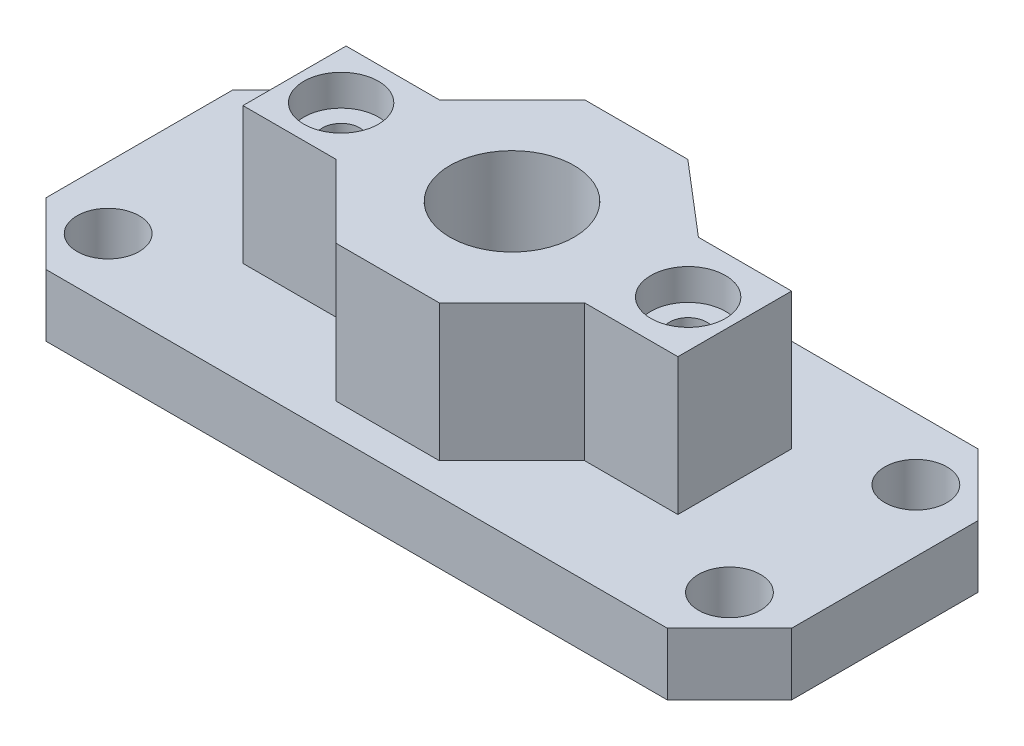
ISO-10303-21;
HEADER;
FILE_DESCRIPTION(('STEP AP214'),'2;1');
FILE_NAME('part.step','',(''),(''),'','','');
FILE_SCHEMA(('AUTOMOTIVE_DESIGN { 1 0 10303 214 1 1 1 1 }'));
ENDSEC;
DATA;
#1=APPLICATION_CONTEXT('core data for automotive mechanical design processes');
#2=APPLICATION_PROTOCOL_DEFINITION('international standard','automotive_design',2000,#1);
#3=PRODUCT_CONTEXT('',#1,'mechanical');
#4=PRODUCT('Part','Part','',(#3));
#5=PRODUCT_RELATED_PRODUCT_CATEGORY('part','',(#4));
#6=PRODUCT_DEFINITION_FORMATION('','',#4);
#7=PRODUCT_DEFINITION_CONTEXT('part definition',#1,'design');
#8=PRODUCT_DEFINITION('design','',#6,#7);
#9=PRODUCT_DEFINITION_SHAPE('','',#8);
#10=(LENGTH_UNIT() NAMED_UNIT(*) SI_UNIT(.MILLI.,.METRE.));
#11=(NAMED_UNIT(*) PLANE_ANGLE_UNIT() SI_UNIT($,.RADIAN.));
#12=(NAMED_UNIT(*) SI_UNIT($,.STERADIAN.) SOLID_ANGLE_UNIT());
#13=UNCERTAINTY_MEASURE_WITH_UNIT(LENGTH_MEASURE(1.E-05),#10,'distance_accuracy_value','');
#14=(GEOMETRIC_REPRESENTATION_CONTEXT(3) GLOBAL_UNCERTAINTY_ASSIGNED_CONTEXT((#13)) GLOBAL_UNIT_ASSIGNED_CONTEXT((#10,
#11,#12)) REPRESENTATION_CONTEXT('',''));
#15=CARTESIAN_POINT('',(0.,0.,0.));
#16=DIRECTION('',(0.,0.,1.));
#17=DIRECTION('',(1.,0.,0.));
#18=AXIS2_PLACEMENT_3D('',#15,#16,#17);
#19=CARTESIAN_POINT('',(120.,10.,50.));
#20=DIRECTION('',(0.,-1.,0.));
#21=DIRECTION('',(0.,0.,-1.));
#22=AXIS2_PLACEMENT_3D('',#19,#20,#21);
#23=PLANE('',#22);
#24=DIRECTION('',(0.,0.,-1.));
#25=VECTOR('',#24,1.);
#26=CARTESIAN_POINT('',(0.,10.,50.));
#27=LINE('',#26,#25);
#28=CARTESIAN_POINT('',(0.,10.,40.));
#29=VERTEX_POINT('',#28);
#30=CARTESIAN_POINT('',(0.,10.,9.99999999999999));
#31=VERTEX_POINT('',#30);
#32=EDGE_CURVE('E246',#29,#31,#27,.T.);
#33=ORIENTED_EDGE('',*,*,#32,.F.);
#34=DIRECTION('',(0.707106781186546,0.,0.70710678118655));
#35=VECTOR('',#34,1.);
#36=CARTESIAN_POINT('',(9.99999999999999,10.,50.));
#37=LINE('',#36,#35);
#38=CARTESIAN_POINT('',(9.99999999999999,10.,50.));
#39=VERTEX_POINT('',#38);
#40=EDGE_CURVE('E294',#29,#39,#37,.T.);
#41=ORIENTED_EDGE('',*,*,#40,.T.);
#42=DIRECTION('',(-1.,0.,0.));
#43=VECTOR('',#42,1.);
#44=CARTESIAN_POINT('',(120.,10.,50.));
#45=LINE('',#44,#43);
#46=CARTESIAN_POINT('',(110.,10.,50.));
#47=VERTEX_POINT('',#46);
#48=EDGE_CURVE('E242',#47,#39,#45,.T.);
#49=ORIENTED_EDGE('',*,*,#48,.F.);
#50=DIRECTION('',(0.707106781186546,0.,-0.707106781186549));
#51=VECTOR('',#50,1.);
#52=CARTESIAN_POINT('',(110.,10.,50.));
#53=LINE('',#52,#51);
#54=CARTESIAN_POINT('',(120.,10.,40.));
#55=VERTEX_POINT('',#54);
#56=EDGE_CURVE('E69',#47,#55,#53,.T.);
#57=ORIENTED_EDGE('',*,*,#56,.T.);
#58=DIRECTION('',(0.,0.,-1.));
#59=VECTOR('',#58,1.);
#60=CARTESIAN_POINT('',(120.,10.,50.));
#61=LINE('',#60,#59);
#62=CARTESIAN_POINT('',(120.,10.,9.99999999999999));
#63=VERTEX_POINT('',#62);
#64=EDGE_CURVE('E254',#55,#63,#61,.T.);
#65=ORIENTED_EDGE('',*,*,#64,.T.);
#66=DIRECTION('',(0.70710678118655,0.,0.707106781186546));
#67=VECTOR('',#66,1.);
#68=CARTESIAN_POINT('',(120.,10.,9.99999999999999));
#69=LINE('',#68,#67);
#70=CARTESIAN_POINT('',(110.,10.,0.));
#71=VERTEX_POINT('',#70);
#72=EDGE_CURVE('E61',#63,#71,#69,.F.);
#73=ORIENTED_EDGE('',*,*,#72,.T.);
#74=DIRECTION('',(-1.,0.,0.));
#75=VECTOR('',#74,1.);
#76=CARTESIAN_POINT('',(120.,10.,0.));
#77=LINE('',#76,#75);
#78=CARTESIAN_POINT('',(10.,10.,0.));
#79=VERTEX_POINT('',#78);
#80=EDGE_CURVE('E244',#71,#79,#77,.T.);
#81=ORIENTED_EDGE('',*,*,#80,.T.);
#82=DIRECTION('',(0.70710678118655,0.,-0.707106781186546));
#83=VECTOR('',#82,1.);
#84=CARTESIAN_POINT('',(0.,10.,9.99999999999999));
#85=LINE('',#84,#83);
#86=EDGE_CURVE('E295',#79,#31,#85,.F.);
#87=ORIENTED_EDGE('',*,*,#86,.T.);
#88=EDGE_LOOP('',(#33,#41,#49,#57,#65,#73,#81,#87));
#89=FACE_BOUND('',#88,.T.);
#90=CARTESIAN_POINT('',(10.,10.,10.));
#91=DIRECTION('',(0.,1.,0.));
#92=DIRECTION('',(0.,0.,1.));
#93=AXIS2_PLACEMENT_3D('',#90,#91,#92);
#94=CIRCLE('',#93,5.);
#95=CARTESIAN_POINT('',(10.,10.,15.));
#96=VERTEX_POINT('',#95);
#97=EDGE_CURVE('E228',#96,#96,#94,.T.);
#98=ORIENTED_EDGE('',*,*,#97,.F.);
#99=EDGE_LOOP('',(#98));
#100=FACE_BOUND('',#99,.T.);
#101=CARTESIAN_POINT('',(110.,10.,40.));
#102=DIRECTION('',(0.,1.,0.));
#103=DIRECTION('',(0.,0.,1.));
#104=AXIS2_PLACEMENT_3D('',#101,#102,#103);
#105=CIRCLE('',#104,5.00000000000001);
#106=CARTESIAN_POINT('',(110.,10.,45.));
#107=VERTEX_POINT('',#106);
#108=EDGE_CURVE('E211',#107,#107,#105,.T.);
#109=ORIENTED_EDGE('',*,*,#108,.F.);
#110=EDGE_LOOP('',(#109));
#111=FACE_BOUND('',#110,.T.);
#112=CARTESIAN_POINT('',(110.,10.,10.));
#113=DIRECTION('',(0.,1.,0.));
#114=DIRECTION('',(0.,0.,1.));
#115=AXIS2_PLACEMENT_3D('',#112,#113,#114);
#116=CIRCLE('',#115,5.);
#117=CARTESIAN_POINT('',(110.,10.,15.));
#118=VERTEX_POINT('',#117);
#119=EDGE_CURVE('E222',#118,#118,#116,.T.);
#120=ORIENTED_EDGE('',*,*,#119,.F.);
#121=EDGE_LOOP('',(#120));
#122=FACE_BOUND('',#121,.T.);
#123=CARTESIAN_POINT('',(10.,10.,40.));
#124=DIRECTION('',(0.,1.,0.));
#125=DIRECTION('',(0.,0.,1.));
#126=AXIS2_PLACEMENT_3D('',#123,#124,#125);
#127=CIRCLE('',#126,5.);
#128=CARTESIAN_POINT('',(10.,10.,45.));
#129=VERTEX_POINT('',#128);
#130=EDGE_CURVE('E230',#129,#129,#127,.T.);
#131=ORIENTED_EDGE('',*,*,#130,.F.);
#132=EDGE_LOOP('',(#131));
#133=FACE_BOUND('',#132,.T.);
#134=DIRECTION('',(0.,0.,1.));
#135=VECTOR('',#134,1.);
#136=CARTESIAN_POINT('',(25.,10.,16.7));
#137=LINE('',#136,#135);
#138=CARTESIAN_POINT('',(25.,10.,16.7));
#139=VERTEX_POINT('',#138);
#140=CARTESIAN_POINT('',(25.,10.,33.3));
#141=VERTEX_POINT('',#140);
#142=EDGE_CURVE('E209',#139,#141,#137,.T.);
#143=ORIENTED_EDGE('',*,*,#142,.F.);
#144=DIRECTION('',(-1.,0.,0.));
#145=VECTOR('',#144,1.);
#146=CARTESIAN_POINT('',(25.,10.,16.7));
#147=LINE('',#146,#145);
#148=CARTESIAN_POINT('',(40.,10.,16.7));
#149=VERTEX_POINT('',#148);
#150=EDGE_CURVE('E210',#149,#139,#147,.T.);
#151=ORIENTED_EDGE('',*,*,#150,.F.);
#152=DIRECTION('',(-0.707106781186548,0.,0.707106781186547));
#153=VECTOR('',#152,1.);
#154=CARTESIAN_POINT('',(40.,10.,16.7));
#155=LINE('',#154,#153);
#156=CARTESIAN_POINT('',(51.7,10.,5.));
#157=VERTEX_POINT('',#156);
#158=EDGE_CURVE('E866',#157,#149,#155,.T.);
#159=ORIENTED_EDGE('',*,*,#158,.F.);
#160=DIRECTION('',(-1.,0.,0.));
#161=VECTOR('',#160,1.);
#162=CARTESIAN_POINT('',(51.7,10.,5.));
#163=LINE('',#162,#161);
#164=CARTESIAN_POINT('',(68.3,10.,5.));
#165=VERTEX_POINT('',#164);
#166=EDGE_CURVE('E861',#165,#157,#163,.T.);
#167=ORIENTED_EDGE('',*,*,#166,.F.);
#168=DIRECTION('',(-0.760173100833643,0.,-0.649720599003114));
#169=VECTOR('',#168,1.);
#170=CARTESIAN_POINT('',(80.,10.,15.));
#171=LINE('',#170,#169);
#172=CARTESIAN_POINT('',(80.,10.,15.));
#173=VERTEX_POINT('',#172);
#174=EDGE_CURVE('E859',#173,#165,#171,.T.);
#175=ORIENTED_EDGE('',*,*,#174,.F.);
#176=DIRECTION('',(-1.,0.,0.));
#177=VECTOR('',#176,1.);
#178=CARTESIAN_POINT('',(95.,10.,15.));
#179=LINE('',#178,#177);
#180=CARTESIAN_POINT('',(95.,10.,15.));
#181=VERTEX_POINT('',#180);
#182=EDGE_CURVE('E857',#181,#173,#179,.T.);
#183=ORIENTED_EDGE('',*,*,#182,.F.);
#184=DIRECTION('',(0.,0.,-1.));
#185=VECTOR('',#184,1.);
#186=CARTESIAN_POINT('',(95.,10.,15.));
#187=LINE('',#186,#185);
#188=CARTESIAN_POINT('',(95.,10.,33.3));
#189=VERTEX_POINT('',#188);
#190=EDGE_CURVE('E852',#189,#181,#187,.T.);
#191=ORIENTED_EDGE('',*,*,#190,.F.);
#192=DIRECTION('',(1.,0.,0.));
#193=VECTOR('',#192,1.);
#194=CARTESIAN_POINT('',(95.,10.,33.3));
#195=LINE('',#194,#193);
#196=CARTESIAN_POINT('',(80.,10.,33.3));
#197=VERTEX_POINT('',#196);
#198=EDGE_CURVE('E853',#197,#189,#195,.T.);
#199=ORIENTED_EDGE('',*,*,#198,.F.);
#200=DIRECTION('',(0.707106781186548,0.,-0.707106781186547));
#201=VECTOR('',#200,1.);
#202=CARTESIAN_POINT('',(80.,10.,33.3));
#203=LINE('',#202,#201);
#204=CARTESIAN_POINT('',(68.3,10.,45.));
#205=VERTEX_POINT('',#204);
#206=EDGE_CURVE('E846',#205,#197,#203,.T.);
#207=ORIENTED_EDGE('',*,*,#206,.F.);
#208=DIRECTION('',(1.,0.,0.));
#209=VECTOR('',#208,1.);
#210=CARTESIAN_POINT('',(51.7,10.,45.));
#211=LINE('',#210,#209);
#212=CARTESIAN_POINT('',(51.7,10.,45.));
#213=VERTEX_POINT('',#212);
#214=EDGE_CURVE('E843',#213,#205,#211,.T.);
#215=ORIENTED_EDGE('',*,*,#214,.F.);
#216=DIRECTION('',(0.707106781186548,0.,0.707106781186547));
#217=VECTOR('',#216,1.);
#218=CARTESIAN_POINT('',(51.7,10.,45.));
#219=LINE('',#218,#217);
#220=CARTESIAN_POINT('',(40.,10.,33.3));
#221=VERTEX_POINT('',#220);
#222=EDGE_CURVE('E845',#221,#213,#219,.T.);
#223=ORIENTED_EDGE('',*,*,#222,.F.);
#224=DIRECTION('',(1.,0.,0.));
#225=VECTOR('',#224,1.);
#226=CARTESIAN_POINT('',(25.,10.,33.3));
#227=LINE('',#226,#225);
#228=EDGE_CURVE('E839',#141,#221,#227,.T.);
#229=ORIENTED_EDGE('',*,*,#228,.F.);
#230=EDGE_LOOP('',(#143,#151,#159,#167,#175,#183,#191,#199,#207,#215,#223,#229));
#231=FACE_BOUND('',#230,.T.);
#232=ADVANCED_FACE('F50',(#89,#100,#111,#122,#133,#231),#23,.F.);
#233=CARTESIAN_POINT('',(0.,10.,50.));
#234=DIRECTION('',(1.,0.,0.));
#235=DIRECTION('',(0.,0.,-1.));
#236=AXIS2_PLACEMENT_3D('',#233,#234,#235);
#237=PLANE('',#236);
#238=DIRECTION('',(0.,0.,-1.));
#239=VECTOR('',#238,1.);
#240=CARTESIAN_POINT('',(0.,0.,50.));
#241=LINE('',#240,#239);
#242=CARTESIAN_POINT('',(0.,0.,40.));
#243=VERTEX_POINT('',#242);
#244=CARTESIAN_POINT('',(0.,0.,9.99999999999999));
#245=VERTEX_POINT('',#244);
#246=EDGE_CURVE('E257',#243,#245,#241,.T.);
#247=ORIENTED_EDGE('',*,*,#246,.F.);
#248=DIRECTION('',(0.,1.,0.));
#249=VECTOR('',#248,1.);
#250=CARTESIAN_POINT('',(0.,10.,40.));
#251=LINE('',#250,#249);
#252=EDGE_CURVE('E286',#243,#29,#251,.T.);
#253=ORIENTED_EDGE('',*,*,#252,.T.);
#254=ORIENTED_EDGE('',*,*,#32,.T.);
#255=DIRECTION('',(0.,-1.,0.));
#256=VECTOR('',#255,1.);
#257=CARTESIAN_POINT('',(0.,10.,9.99999999999999));
#258=LINE('',#257,#256);
#259=EDGE_CURVE('E284',#31,#245,#258,.T.);
#260=ORIENTED_EDGE('',*,*,#259,.T.);
#261=EDGE_LOOP('',(#247,#253,#254,#260));
#262=FACE_BOUND('',#261,.T.);
#263=ADVANCED_FACE('F321',(#262),#237,.F.);
#264=CARTESIAN_POINT('',(0.,0.,50.));
#265=DIRECTION('',(0.,1.,0.));
#266=DIRECTION('',(0.,0.,1.));
#267=AXIS2_PLACEMENT_3D('',#264,#265,#266);
#268=PLANE('',#267);
#269=CARTESIAN_POINT('',(10.,0.,40.));
#270=DIRECTION('',(0.,1.,0.));
#271=DIRECTION('',(0.,0.,1.));
#272=AXIS2_PLACEMENT_3D('',#269,#270,#271);
#273=CIRCLE('',#272,5.);
#274=CARTESIAN_POINT('',(10.,0.,45.));
#275=VERTEX_POINT('',#274);
#276=EDGE_CURVE('E224',#275,#275,#273,.T.);
#277=ORIENTED_EDGE('',*,*,#276,.T.);
#278=EDGE_LOOP('',(#277));
#279=FACE_BOUND('',#278,.T.);
#280=CARTESIAN_POINT('',(110.,0.,10.));
#281=DIRECTION('',(0.,1.,0.));
#282=DIRECTION('',(0.,0.,1.));
#283=AXIS2_PLACEMENT_3D('',#280,#281,#282);
#284=CIRCLE('',#283,5.);
#285=CARTESIAN_POINT('',(110.,0.,15.));
#286=VERTEX_POINT('',#285);
#287=EDGE_CURVE('E229',#286,#286,#284,.T.);
#288=ORIENTED_EDGE('',*,*,#287,.T.);
#289=EDGE_LOOP('',(#288));
#290=FACE_BOUND('',#289,.T.);
#291=CARTESIAN_POINT('',(110.,0.,40.));
#292=DIRECTION('',(0.,1.,0.));
#293=DIRECTION('',(0.,0.,1.));
#294=AXIS2_PLACEMENT_3D('',#291,#292,#293);
#295=CIRCLE('',#294,5.00000000000001);
#296=CARTESIAN_POINT('',(110.,0.,45.));
#297=VERTEX_POINT('',#296);
#298=EDGE_CURVE('E212',#297,#297,#295,.T.);
#299=ORIENTED_EDGE('',*,*,#298,.T.);
#300=EDGE_LOOP('',(#299));
#301=FACE_BOUND('',#300,.T.);
#302=CARTESIAN_POINT('',(10.,0.,10.));
#303=DIRECTION('',(0.,1.,0.));
#304=DIRECTION('',(0.,0.,1.));
#305=AXIS2_PLACEMENT_3D('',#302,#303,#304);
#306=CIRCLE('',#305,5.);
#307=CARTESIAN_POINT('',(10.,0.,15.));
#308=VERTEX_POINT('',#307);
#309=EDGE_CURVE('E234',#308,#308,#306,.T.);
#310=ORIENTED_EDGE('',*,*,#309,.T.);
#311=EDGE_LOOP('',(#310));
#312=FACE_BOUND('',#311,.T.);
#313=DIRECTION('',(1.,0.,0.));
#314=VECTOR('',#313,1.);
#315=CARTESIAN_POINT('',(0.,0.,50.));
#316=LINE('',#315,#314);
#317=CARTESIAN_POINT('',(9.99999999999999,0.,50.));
#318=VERTEX_POINT('',#317);
#319=CARTESIAN_POINT('',(110.,0.,50.));
#320=VERTEX_POINT('',#319);
#321=EDGE_CURVE('E243',#318,#320,#316,.T.);
#322=ORIENTED_EDGE('',*,*,#321,.F.);
#323=DIRECTION('',(-0.707106781186546,0.,-0.70710678118655));
#324=VECTOR('',#323,1.);
#325=CARTESIAN_POINT('',(9.99999999999999,0.,50.));
#326=LINE('',#325,#324);
#327=EDGE_CURVE('E281',#318,#243,#326,.T.);
#328=ORIENTED_EDGE('',*,*,#327,.T.);
#329=ORIENTED_EDGE('',*,*,#246,.T.);
#330=DIRECTION('',(-0.70710678118655,0.,0.707106781186546));
#331=VECTOR('',#330,1.);
#332=CARTESIAN_POINT('',(0.,0.,9.99999999999999));
#333=LINE('',#332,#331);
#334=CARTESIAN_POINT('',(10.,0.,0.));
#335=VERTEX_POINT('',#334);
#336=EDGE_CURVE('E283',#245,#335,#333,.F.);
#337=ORIENTED_EDGE('',*,*,#336,.T.);
#338=DIRECTION('',(1.,0.,0.));
#339=VECTOR('',#338,1.);
#340=CARTESIAN_POINT('',(0.,0.,0.));
#341=LINE('',#340,#339);
#342=CARTESIAN_POINT('',(110.,0.,0.));
#343=VERTEX_POINT('',#342);
#344=EDGE_CURVE('E236',#335,#343,#341,.T.);
#345=ORIENTED_EDGE('',*,*,#344,.T.);
#346=DIRECTION('',(-0.70710678118655,0.,-0.707106781186546));
#347=VECTOR('',#346,1.);
#348=CARTESIAN_POINT('',(120.,0.,9.99999999999999));
#349=LINE('',#348,#347);
#350=CARTESIAN_POINT('',(120.,0.,9.99999999999999));
#351=VERTEX_POINT('',#350);
#352=EDGE_CURVE('E276',#343,#351,#349,.F.);
#353=ORIENTED_EDGE('',*,*,#352,.T.);
#354=DIRECTION('',(0.,0.,-1.));
#355=VECTOR('',#354,1.);
#356=CARTESIAN_POINT('',(120.,0.,50.));
#357=LINE('',#356,#355);
#358=CARTESIAN_POINT('',(120.,0.,40.));
#359=VERTEX_POINT('',#358);
#360=EDGE_CURVE('E260',#359,#351,#357,.T.);
#361=ORIENTED_EDGE('',*,*,#360,.F.);
#362=DIRECTION('',(-0.707106781186546,0.,0.707106781186549));
#363=VECTOR('',#362,1.);
#364=CARTESIAN_POINT('',(110.,0.,50.));
#365=LINE('',#364,#363);
#366=EDGE_CURVE('E280',#359,#320,#365,.T.);
#367=ORIENTED_EDGE('',*,*,#366,.T.);
#368=EDGE_LOOP('',(#322,#328,#329,#337,#345,#353,#361,#367));
#369=FACE_BOUND('',#368,.T.);
#370=ADVANCED_FACE('F307',(#279,#290,#301,#312,#369),#268,.F.);
#371=CARTESIAN_POINT('',(120.,0.,50.));
#372=DIRECTION('',(-1.,0.,0.));
#373=DIRECTION('',(0.,0.,1.));
#374=AXIS2_PLACEMENT_3D('',#371,#372,#373);
#375=PLANE('',#374);
#376=ORIENTED_EDGE('',*,*,#360,.T.);
#377=DIRECTION('',(0.,1.,0.));
#378=VECTOR('',#377,1.);
#379=CARTESIAN_POINT('',(120.,0.,9.99999999999999));
#380=LINE('',#379,#378);
#381=EDGE_CURVE('E11',#351,#63,#380,.T.);
#382=ORIENTED_EDGE('',*,*,#381,.T.);
#383=ORIENTED_EDGE('',*,*,#64,.F.);
#384=DIRECTION('',(0.,-1.,0.));
#385=VECTOR('',#384,1.);
#386=CARTESIAN_POINT('',(120.,0.,40.));
#387=LINE('',#386,#385);
#388=EDGE_CURVE('E57',#55,#359,#387,.T.);
#389=ORIENTED_EDGE('',*,*,#388,.T.);
#390=EDGE_LOOP('',(#376,#382,#383,#389));
#391=FACE_BOUND('',#390,.T.);
#392=ADVANCED_FACE('F305',(#391),#375,.F.);
#393=CARTESIAN_POINT('',(0.,0.,50.));
#394=DIRECTION('',(0.,0.,1.));
#395=DIRECTION('',(1.,0.,0.));
#396=AXIS2_PLACEMENT_3D('',#393,#394,#395);
#397=PLANE('',#396);
#398=ORIENTED_EDGE('',*,*,#48,.T.);
#399=DIRECTION('',(0.,-1.,0.));
#400=VECTOR('',#399,1.);
#401=CARTESIAN_POINT('',(9.99999999999999,0.,50.));
#402=LINE('',#401,#400);
#403=EDGE_CURVE('E273',#39,#318,#402,.T.);
#404=ORIENTED_EDGE('',*,*,#403,.T.);
#405=ORIENTED_EDGE('',*,*,#321,.T.);
#406=DIRECTION('',(0.,1.,0.));
#407=VECTOR('',#406,1.);
#408=CARTESIAN_POINT('',(110.,10.,50.));
#409=LINE('',#408,#407);
#410=EDGE_CURVE('E263',#320,#47,#409,.T.);
#411=ORIENTED_EDGE('',*,*,#410,.T.);
#412=EDGE_LOOP('',(#398,#404,#405,#411));
#413=FACE_BOUND('',#412,.T.);
#414=ADVANCED_FACE('F313',(#413),#397,.T.);
#415=CARTESIAN_POINT('',(0.,0.,0.));
#416=DIRECTION('',(0.,0.,1.));
#417=DIRECTION('',(1.,0.,0.));
#418=AXIS2_PLACEMENT_3D('',#415,#416,#417);
#419=PLANE('',#418);
#420=ORIENTED_EDGE('',*,*,#344,.F.);
#421=DIRECTION('',(0.,1.,0.));
#422=VECTOR('',#421,1.);
#423=CARTESIAN_POINT('',(10.,0.,0.));
#424=LINE('',#423,#422);
#425=EDGE_CURVE('E296',#335,#79,#424,.T.);
#426=ORIENTED_EDGE('',*,*,#425,.T.);
#427=ORIENTED_EDGE('',*,*,#80,.F.);
#428=DIRECTION('',(0.,-1.,0.));
#429=VECTOR('',#428,1.);
#430=CARTESIAN_POINT('',(110.,0.,0.));
#431=LINE('',#430,#429);
#432=EDGE_CURVE('E298',#71,#343,#431,.T.);
#433=ORIENTED_EDGE('',*,*,#432,.T.);
#434=EDGE_LOOP('',(#420,#426,#427,#433));
#435=FACE_BOUND('',#434,.T.);
#436=ADVANCED_FACE('F328',(#435),#419,.F.);
#437=CARTESIAN_POINT('',(10.,0.,10.));
#438=DIRECTION('',(0.,1.,0.));
#439=DIRECTION('',(0.,0.,1.));
#440=AXIS2_PLACEMENT_3D('',#437,#438,#439);
#441=CYLINDRICAL_SURFACE('',#440,5.);
#442=ORIENTED_EDGE('',*,*,#309,.F.);
#443=EDGE_LOOP('',(#442));
#444=FACE_BOUND('',#443,.T.);
#445=ORIENTED_EDGE('',*,*,#97,.T.);
#446=EDGE_LOOP('',(#445));
#447=FACE_BOUND('',#446,.T.);
#448=ADVANCED_FACE('F448',(#444,#447),#441,.F.);
#449=CARTESIAN_POINT('',(110.,0.,40.));
#450=DIRECTION('',(0.,1.,0.));
#451=DIRECTION('',(0.,0.,1.));
#452=AXIS2_PLACEMENT_3D('',#449,#450,#451);
#453=CYLINDRICAL_SURFACE('',#452,5.00000000000001);
#454=ORIENTED_EDGE('',*,*,#298,.F.);
#455=EDGE_LOOP('',(#454));
#456=FACE_BOUND('',#455,.T.);
#457=ORIENTED_EDGE('',*,*,#108,.T.);
#458=EDGE_LOOP('',(#457));
#459=FACE_BOUND('',#458,.T.);
#460=ADVANCED_FACE('F445',(#456,#459),#453,.F.);
#461=CARTESIAN_POINT('',(110.,0.,10.));
#462=DIRECTION('',(0.,1.,0.));
#463=DIRECTION('',(0.,0.,1.));
#464=AXIS2_PLACEMENT_3D('',#461,#462,#463);
#465=CYLINDRICAL_SURFACE('',#464,5.);
#466=ORIENTED_EDGE('',*,*,#287,.F.);
#467=EDGE_LOOP('',(#466));
#468=FACE_BOUND('',#467,.T.);
#469=ORIENTED_EDGE('',*,*,#119,.T.);
#470=EDGE_LOOP('',(#469));
#471=FACE_BOUND('',#470,.T.);
#472=ADVANCED_FACE('F443',(#468,#471),#465,.F.);
#473=CARTESIAN_POINT('',(10.,0.,40.));
#474=DIRECTION('',(0.,1.,0.));
#475=DIRECTION('',(0.,0.,1.));
#476=AXIS2_PLACEMENT_3D('',#473,#474,#475);
#477=CYLINDRICAL_SURFACE('',#476,5.);
#478=ORIENTED_EDGE('',*,*,#276,.F.);
#479=EDGE_LOOP('',(#478));
#480=FACE_BOUND('',#479,.T.);
#481=ORIENTED_EDGE('',*,*,#130,.T.);
#482=EDGE_LOOP('',(#481));
#483=FACE_BOUND('',#482,.T.);
#484=ADVANCED_FACE('F442',(#480,#483),#477,.F.);
#485=CARTESIAN_POINT('',(25.,32.,16.7));
#486=DIRECTION('',(1.,0.,0.));
#487=DIRECTION('',(0.,0.,-1.));
#488=AXIS2_PLACEMENT_3D('',#485,#486,#487);
#489=PLANE('',#488);
#490=ORIENTED_EDGE('',*,*,#142,.T.);
#491=DIRECTION('',(0.,-1.,0.));
#492=VECTOR('',#491,1.);
#493=CARTESIAN_POINT('',(25.,32.,33.3));
#494=LINE('',#493,#492);
#495=CARTESIAN_POINT('',(25.,32.,33.3));
#496=VERTEX_POINT('',#495);
#497=EDGE_CURVE('E193',#496,#141,#494,.T.);
#498=ORIENTED_EDGE('',*,*,#497,.F.);
#499=DIRECTION('',(0.,0.,1.));
#500=VECTOR('',#499,1.);
#501=CARTESIAN_POINT('',(25.,32.,16.7));
#502=LINE('',#501,#500);
#503=CARTESIAN_POINT('',(25.,32.,16.7));
#504=VERTEX_POINT('',#503);
#505=EDGE_CURVE('E196',#504,#496,#502,.T.);
#506=ORIENTED_EDGE('',*,*,#505,.F.);
#507=DIRECTION('',(0.,-1.,0.));
#508=VECTOR('',#507,1.);
#509=CARTESIAN_POINT('',(25.,32.,16.7));
#510=LINE('',#509,#508);
#511=EDGE_CURVE('E836',#504,#139,#510,.T.);
#512=ORIENTED_EDGE('',*,*,#511,.T.);
#513=EDGE_LOOP('',(#490,#498,#506,#512));
#514=FACE_BOUND('',#513,.T.);
#515=ADVANCED_FACE('F207',(#514),#489,.F.);
#516=CARTESIAN_POINT('',(25.,32.,33.3));
#517=DIRECTION('',(0.,0.,-1.));
#518=DIRECTION('',(-1.,0.,0.));
#519=AXIS2_PLACEMENT_3D('',#516,#517,#518);
#520=PLANE('',#519);
#521=ORIENTED_EDGE('',*,*,#228,.T.);
#522=DIRECTION('',(0.,-1.,0.));
#523=VECTOR('',#522,1.);
#524=CARTESIAN_POINT('',(40.,32.,33.3));
#525=LINE('',#524,#523);
#526=CARTESIAN_POINT('',(40.,32.,33.3));
#527=VERTEX_POINT('',#526);
#528=EDGE_CURVE('E192',#527,#221,#525,.T.);
#529=ORIENTED_EDGE('',*,*,#528,.F.);
#530=DIRECTION('',(1.,0.,0.));
#531=VECTOR('',#530,1.);
#532=CARTESIAN_POINT('',(25.,32.,33.3));
#533=LINE('',#532,#531);
#534=EDGE_CURVE('E188',#496,#527,#533,.T.);
#535=ORIENTED_EDGE('',*,*,#534,.F.);
#536=ORIENTED_EDGE('',*,*,#497,.T.);
#537=EDGE_LOOP('',(#521,#529,#535,#536));
#538=FACE_BOUND('',#537,.T.);
#539=ADVANCED_FACE('F187',(#538),#520,.F.);
#540=CARTESIAN_POINT('',(51.7,32.,45.));
#541=DIRECTION('',(0.707106781186547,0.,-0.707106781186548));
#542=DIRECTION('',(-0.707106781186548,0.,-0.707106781186547));
#543=AXIS2_PLACEMENT_3D('',#540,#541,#542);
#544=PLANE('',#543);
#545=ORIENTED_EDGE('',*,*,#222,.T.);
#546=DIRECTION('',(0.,-1.,0.));
#547=VECTOR('',#546,1.);
#548=CARTESIAN_POINT('',(51.7,32.,45.));
#549=LINE('',#548,#547);
#550=CARTESIAN_POINT('',(51.7,32.,45.));
#551=VERTEX_POINT('',#550);
#552=EDGE_CURVE('E216',#551,#213,#549,.T.);
#553=ORIENTED_EDGE('',*,*,#552,.F.);
#554=DIRECTION('',(0.707106781186548,0.,0.707106781186547));
#555=VECTOR('',#554,1.);
#556=CARTESIAN_POINT('',(51.7,32.,45.));
#557=LINE('',#556,#555);
#558=EDGE_CURVE('E197',#527,#551,#557,.T.);
#559=ORIENTED_EDGE('',*,*,#558,.F.);
#560=ORIENTED_EDGE('',*,*,#528,.T.);
#561=EDGE_LOOP('',(#545,#553,#559,#560));
#562=FACE_BOUND('',#561,.T.);
#563=ADVANCED_FACE('F435',(#562),#544,.F.);
#564=CARTESIAN_POINT('',(51.7,32.,45.));
#565=DIRECTION('',(0.,0.,-1.));
#566=DIRECTION('',(-1.,0.,0.));
#567=AXIS2_PLACEMENT_3D('',#564,#565,#566);
#568=PLANE('',#567);
#569=ORIENTED_EDGE('',*,*,#214,.T.);
#570=DIRECTION('',(0.,-1.,0.));
#571=VECTOR('',#570,1.);
#572=CARTESIAN_POINT('',(68.3,32.,45.));
#573=LINE('',#572,#571);
#574=CARTESIAN_POINT('',(68.3,32.,45.));
#575=VERTEX_POINT('',#574);
#576=EDGE_CURVE('E891',#575,#205,#573,.T.);
#577=ORIENTED_EDGE('',*,*,#576,.F.);
#578=DIRECTION('',(1.,0.,0.));
#579=VECTOR('',#578,1.);
#580=CARTESIAN_POINT('',(51.7,32.,45.));
#581=LINE('',#580,#579);
#582=EDGE_CURVE('E821',#551,#575,#581,.T.);
#583=ORIENTED_EDGE('',*,*,#582,.F.);
#584=ORIENTED_EDGE('',*,*,#552,.T.);
#585=EDGE_LOOP('',(#569,#577,#583,#584));
#586=FACE_BOUND('',#585,.T.);
#587=ADVANCED_FACE('F428',(#586),#568,.F.);
#588=CARTESIAN_POINT('',(80.,32.,33.3));
#589=DIRECTION('',(-0.707106781186547,0.,-0.707106781186548));
#590=DIRECTION('',(-0.707106781186548,0.,0.707106781186547));
#591=AXIS2_PLACEMENT_3D('',#588,#589,#590);
#592=PLANE('',#591);
#593=ORIENTED_EDGE('',*,*,#206,.T.);
#594=DIRECTION('',(0.,-1.,0.));
#595=VECTOR('',#594,1.);
#596=CARTESIAN_POINT('',(80.,32.,33.3));
#597=LINE('',#596,#595);
#598=CARTESIAN_POINT('',(80.,32.,33.3));
#599=VERTEX_POINT('',#598);
#600=EDGE_CURVE('E889',#599,#197,#597,.T.);
#601=ORIENTED_EDGE('',*,*,#600,.F.);
#602=DIRECTION('',(0.707106781186548,0.,-0.707106781186547));
#603=VECTOR('',#602,1.);
#604=CARTESIAN_POINT('',(80.,32.,33.3));
#605=LINE('',#604,#603);
#606=EDGE_CURVE('E822',#575,#599,#605,.T.);
#607=ORIENTED_EDGE('',*,*,#606,.F.);
#608=ORIENTED_EDGE('',*,*,#576,.T.);
#609=EDGE_LOOP('',(#593,#601,#607,#608));
#610=FACE_BOUND('',#609,.T.);
#611=ADVANCED_FACE('F424',(#610),#592,.F.);
#612=CARTESIAN_POINT('',(95.,32.,33.3));
#613=DIRECTION('',(0.,0.,-1.));
#614=DIRECTION('',(-1.,0.,0.));
#615=AXIS2_PLACEMENT_3D('',#612,#613,#614);
#616=PLANE('',#615);
#617=ORIENTED_EDGE('',*,*,#198,.T.);
#618=DIRECTION('',(0.,-1.,0.));
#619=VECTOR('',#618,1.);
#620=CARTESIAN_POINT('',(95.,32.,33.3));
#621=LINE('',#620,#619);
#622=CARTESIAN_POINT('',(95.,32.,33.3));
#623=VERTEX_POINT('',#622);
#624=EDGE_CURVE('E890',#623,#189,#621,.T.);
#625=ORIENTED_EDGE('',*,*,#624,.F.);
#626=DIRECTION('',(1.,0.,0.));
#627=VECTOR('',#626,1.);
#628=CARTESIAN_POINT('',(95.,32.,33.3));
#629=LINE('',#628,#627);
#630=EDGE_CURVE('E824',#599,#623,#629,.T.);
#631=ORIENTED_EDGE('',*,*,#630,.F.);
#632=ORIENTED_EDGE('',*,*,#600,.T.);
#633=EDGE_LOOP('',(#617,#625,#631,#632));
#634=FACE_BOUND('',#633,.T.);
#635=ADVANCED_FACE('F419',(#634),#616,.F.);
#636=CARTESIAN_POINT('',(95.,32.,15.));
#637=DIRECTION('',(-1.,0.,0.));
#638=DIRECTION('',(0.,0.,1.));
#639=AXIS2_PLACEMENT_3D('',#636,#637,#638);
#640=PLANE('',#639);
#641=ORIENTED_EDGE('',*,*,#190,.T.);
#642=DIRECTION('',(0.,-1.,0.));
#643=VECTOR('',#642,1.);
#644=CARTESIAN_POINT('',(95.,32.,15.));
#645=LINE('',#644,#643);
#646=CARTESIAN_POINT('',(95.,32.,15.));
#647=VERTEX_POINT('',#646);
#648=EDGE_CURVE('E881',#647,#181,#645,.T.);
#649=ORIENTED_EDGE('',*,*,#648,.F.);
#650=DIRECTION('',(0.,0.,-1.));
#651=VECTOR('',#650,1.);
#652=CARTESIAN_POINT('',(95.,32.,15.));
#653=LINE('',#652,#651);
#654=EDGE_CURVE('E830',#623,#647,#653,.T.);
#655=ORIENTED_EDGE('',*,*,#654,.F.);
#656=ORIENTED_EDGE('',*,*,#624,.T.);
#657=EDGE_LOOP('',(#641,#649,#655,#656));
#658=FACE_BOUND('',#657,.T.);
#659=ADVANCED_FACE('F418',(#658),#640,.F.);
#660=CARTESIAN_POINT('',(95.,32.,15.));
#661=DIRECTION('',(0.,0.,1.));
#662=DIRECTION('',(1.,0.,0.));
#663=AXIS2_PLACEMENT_3D('',#660,#661,#662);
#664=PLANE('',#663);
#665=ORIENTED_EDGE('',*,*,#182,.T.);
#666=DIRECTION('',(0.,-1.,0.));
#667=VECTOR('',#666,1.);
#668=CARTESIAN_POINT('',(80.,32.,15.));
#669=LINE('',#668,#667);
#670=CARTESIAN_POINT('',(80.,32.,15.));
#671=VERTEX_POINT('',#670);
#672=EDGE_CURVE('E882',#671,#173,#669,.T.);
#673=ORIENTED_EDGE('',*,*,#672,.F.);
#674=DIRECTION('',(-1.,0.,0.));
#675=VECTOR('',#674,1.);
#676=CARTESIAN_POINT('',(95.,32.,15.));
#677=LINE('',#676,#675);
#678=EDGE_CURVE('E826',#647,#671,#677,.T.);
#679=ORIENTED_EDGE('',*,*,#678,.F.);
#680=ORIENTED_EDGE('',*,*,#648,.T.);
#681=EDGE_LOOP('',(#665,#673,#679,#680));
#682=FACE_BOUND('',#681,.T.);
#683=ADVANCED_FACE('F415',(#682),#664,.F.);
#684=CARTESIAN_POINT('',(80.,32.,15.));
#685=DIRECTION('',(-0.649720599003114,0.,0.760173100833643));
#686=DIRECTION('',(0.760173100833643,0.,0.649720599003114));
#687=AXIS2_PLACEMENT_3D('',#684,#685,#686);
#688=PLANE('',#687);
#689=ORIENTED_EDGE('',*,*,#174,.T.);
#690=DIRECTION('',(0.,-1.,0.));
#691=VECTOR('',#690,1.);
#692=CARTESIAN_POINT('',(68.3,32.,5.));
#693=LINE('',#692,#691);
#694=CARTESIAN_POINT('',(68.3,32.,5.));
#695=VERTEX_POINT('',#694);
#696=EDGE_CURVE('E877',#695,#165,#693,.T.);
#697=ORIENTED_EDGE('',*,*,#696,.F.);
#698=DIRECTION('',(-0.760173100833643,0.,-0.649720599003114));
#699=VECTOR('',#698,1.);
#700=CARTESIAN_POINT('',(80.,32.,15.));
#701=LINE('',#700,#699);
#702=EDGE_CURVE('E833',#671,#695,#701,.T.);
#703=ORIENTED_EDGE('',*,*,#702,.F.);
#704=ORIENTED_EDGE('',*,*,#672,.T.);
#705=EDGE_LOOP('',(#689,#697,#703,#704));
#706=FACE_BOUND('',#705,.T.);
#707=ADVANCED_FACE('F406',(#706),#688,.F.);
#708=CARTESIAN_POINT('',(51.7,32.,5.));
#709=DIRECTION('',(0.,0.,1.));
#710=DIRECTION('',(1.,0.,0.));
#711=AXIS2_PLACEMENT_3D('',#708,#709,#710);
#712=PLANE('',#711);
#713=ORIENTED_EDGE('',*,*,#166,.T.);
#714=DIRECTION('',(0.,-1.,0.));
#715=VECTOR('',#714,1.);
#716=CARTESIAN_POINT('',(51.7,32.,5.));
#717=LINE('',#716,#715);
#718=CARTESIAN_POINT('',(51.7,32.,5.));
#719=VERTEX_POINT('',#718);
#720=EDGE_CURVE('E874',#719,#157,#717,.T.);
#721=ORIENTED_EDGE('',*,*,#720,.F.);
#722=DIRECTION('',(-1.,0.,0.));
#723=VECTOR('',#722,1.);
#724=CARTESIAN_POINT('',(51.7,32.,5.));
#725=LINE('',#724,#723);
#726=EDGE_CURVE('E831',#695,#719,#725,.T.);
#727=ORIENTED_EDGE('',*,*,#726,.F.);
#728=ORIENTED_EDGE('',*,*,#696,.T.);
#729=EDGE_LOOP('',(#713,#721,#727,#728));
#730=FACE_BOUND('',#729,.T.);
#731=ADVANCED_FACE('F404',(#730),#712,.F.);
#732=CARTESIAN_POINT('',(40.,32.,16.7));
#733=DIRECTION('',(0.707106781186547,0.,0.707106781186548));
#734=DIRECTION('',(0.707106781186548,0.,-0.707106781186547));
#735=AXIS2_PLACEMENT_3D('',#732,#733,#734);
#736=PLANE('',#735);
#737=ORIENTED_EDGE('',*,*,#158,.T.);
#738=DIRECTION('',(0.,-1.,0.));
#739=VECTOR('',#738,1.);
#740=CARTESIAN_POINT('',(40.,32.,16.7));
#741=LINE('',#740,#739);
#742=CARTESIAN_POINT('',(40.,32.,16.7));
#743=VERTEX_POINT('',#742);
#744=EDGE_CURVE('E875',#743,#149,#741,.T.);
#745=ORIENTED_EDGE('',*,*,#744,.F.);
#746=DIRECTION('',(-0.707106781186548,0.,0.707106781186547));
#747=VECTOR('',#746,1.);
#748=CARTESIAN_POINT('',(40.,32.,16.7));
#749=LINE('',#748,#747);
#750=EDGE_CURVE('E834',#719,#743,#749,.T.);
#751=ORIENTED_EDGE('',*,*,#750,.F.);
#752=ORIENTED_EDGE('',*,*,#720,.T.);
#753=EDGE_LOOP('',(#737,#745,#751,#752));
#754=FACE_BOUND('',#753,.T.);
#755=ADVANCED_FACE('F399',(#754),#736,.F.);
#756=CARTESIAN_POINT('',(25.,32.,16.7));
#757=DIRECTION('',(0.,0.,1.));
#758=DIRECTION('',(1.,0.,0.));
#759=AXIS2_PLACEMENT_3D('',#756,#757,#758);
#760=PLANE('',#759);
#761=ORIENTED_EDGE('',*,*,#150,.T.);
#762=ORIENTED_EDGE('',*,*,#511,.F.);
#763=DIRECTION('',(-1.,0.,0.));
#764=VECTOR('',#763,1.);
#765=CARTESIAN_POINT('',(25.,32.,16.7));
#766=LINE('',#765,#764);
#767=EDGE_CURVE('E201',#743,#504,#766,.T.);
#768=ORIENTED_EDGE('',*,*,#767,.F.);
#769=ORIENTED_EDGE('',*,*,#744,.T.);
#770=EDGE_LOOP('',(#761,#762,#768,#769));
#771=FACE_BOUND('',#770,.T.);
#772=ADVANCED_FACE('F398',(#771),#760,.F.);
#773=CARTESIAN_POINT('',(0.,32.,0.));
#774=DIRECTION('',(0.,1.,0.));
#775=DIRECTION('',(0.,0.,1.));
#776=AXIS2_PLACEMENT_3D('',#773,#774,#775);
#777=PLANE('',#776);
#778=CARTESIAN_POINT('',(32.5,32.,25.));
#779=DIRECTION('',(0.,1.,0.));
#780=DIRECTION('',(0.,0.,1.));
#781=AXIS2_PLACEMENT_3D('',#778,#779,#780);
#782=CIRCLE('',#781,6.);
#783=CARTESIAN_POINT('',(32.5,32.,31.));
#784=VERTEX_POINT('',#783);
#785=EDGE_CURVE('E925',#784,#784,#782,.T.);
#786=ORIENTED_EDGE('',*,*,#785,.F.);
#787=EDGE_LOOP('',(#786));
#788=FACE_BOUND('',#787,.T.);
#789=CARTESIAN_POINT('',(87.5,32.,24.15));
#790=DIRECTION('',(0.,1.,0.));
#791=DIRECTION('',(0.,0.,1.));
#792=AXIS2_PLACEMENT_3D('',#789,#790,#791);
#793=CIRCLE('',#792,6.);
#794=CARTESIAN_POINT('',(87.5,32.,30.15));
#795=VERTEX_POINT('',#794);
#796=EDGE_CURVE('E814',#795,#795,#793,.T.);
#797=ORIENTED_EDGE('',*,*,#796,.F.);
#798=EDGE_LOOP('',(#797));
#799=FACE_BOUND('',#798,.T.);
#800=CARTESIAN_POINT('',(60.,32.,25.));
#801=DIRECTION('',(0.,1.,0.));
#802=DIRECTION('',(0.,0.,1.));
#803=AXIS2_PLACEMENT_3D('',#800,#801,#802);
#804=CIRCLE('',#803,9.99999999999999);
#805=CARTESIAN_POINT('',(60.,32.,35.));
#806=VERTEX_POINT('',#805);
#807=EDGE_CURVE('E810',#806,#806,#804,.T.);
#808=ORIENTED_EDGE('',*,*,#807,.F.);
#809=EDGE_LOOP('',(#808));
#810=FACE_BOUND('',#809,.T.);
#811=ORIENTED_EDGE('',*,*,#505,.T.);
#812=ORIENTED_EDGE('',*,*,#534,.T.);
#813=ORIENTED_EDGE('',*,*,#558,.T.);
#814=ORIENTED_EDGE('',*,*,#582,.T.);
#815=ORIENTED_EDGE('',*,*,#606,.T.);
#816=ORIENTED_EDGE('',*,*,#630,.T.);
#817=ORIENTED_EDGE('',*,*,#654,.T.);
#818=ORIENTED_EDGE('',*,*,#678,.T.);
#819=ORIENTED_EDGE('',*,*,#702,.T.);
#820=ORIENTED_EDGE('',*,*,#726,.T.);
#821=ORIENTED_EDGE('',*,*,#750,.T.);
#822=ORIENTED_EDGE('',*,*,#767,.T.);
#823=EDGE_LOOP('',(#811,#812,#813,#814,#815,#816,#817,#818,#819,#820,#821,#822));
#824=FACE_BOUND('',#823,.T.);
#825=ADVANCED_FACE('F203',(#788,#799,#810,#824),#777,.T.);
#826=CARTESIAN_POINT('',(60.,10.,25.));
#827=DIRECTION('',(0.,1.,0.));
#828=DIRECTION('',(0.,0.,1.));
#829=AXIS2_PLACEMENT_3D('',#826,#827,#828);
#830=CYLINDRICAL_SURFACE('',#829,9.99999999999999);
#831=CARTESIAN_POINT('',(60.,10.,25.));
#832=DIRECTION('',(0.,1.,0.));
#833=DIRECTION('',(0.,0.,1.));
#834=AXIS2_PLACEMENT_3D('',#831,#832,#833);
#835=CIRCLE('',#834,9.99999999999999);
#836=CARTESIAN_POINT('',(60.,10.,35.));
#837=VERTEX_POINT('',#836);
#838=EDGE_CURVE('E807',#837,#837,#835,.T.);
#839=ORIENTED_EDGE('',*,*,#838,.F.);
#840=EDGE_LOOP('',(#839));
#841=FACE_BOUND('',#840,.T.);
#842=ORIENTED_EDGE('',*,*,#807,.T.);
#843=EDGE_LOOP('',(#842));
#844=FACE_BOUND('',#843,.T.);
#845=ADVANCED_FACE('F386',(#841,#844),#830,.F.);
#846=CARTESIAN_POINT('',(60.,10.,25.));
#847=DIRECTION('',(0.,1.,0.));
#848=DIRECTION('',(0.,0.,1.));
#849=AXIS2_PLACEMENT_3D('',#846,#847,#848);
#850=PLANE('',#849);
#851=ORIENTED_EDGE('',*,*,#838,.T.);
#852=EDGE_LOOP('',(#851));
#853=FACE_BOUND('',#852,.T.);
#854=ADVANCED_FACE('F384',(#853),#850,.T.);
#855=CARTESIAN_POINT('',(32.5,27.,25.));
#856=DIRECTION('',(0.,1.,0.));
#857=DIRECTION('',(0.,0.,1.));
#858=AXIS2_PLACEMENT_3D('',#855,#856,#857);
#859=PLANE('',#858);
#860=CARTESIAN_POINT('',(32.5,27.,25.));
#861=DIRECTION('',(0.,1.,0.));
#862=DIRECTION('',(0.,0.,1.));
#863=AXIS2_PLACEMENT_3D('',#860,#861,#862);
#864=CIRCLE('',#863,6.);
#865=CARTESIAN_POINT('',(32.5,27.,31.));
#866=VERTEX_POINT('',#865);
#867=EDGE_CURVE('E268',#866,#866,#864,.T.);
#868=ORIENTED_EDGE('',*,*,#867,.T.);
#869=EDGE_LOOP('',(#868));
#870=FACE_BOUND('',#869,.T.);
#871=CARTESIAN_POINT('',(32.5,27.,25.));
#872=DIRECTION('',(0.,1.,0.));
#873=DIRECTION('',(0.,0.,1.));
#874=AXIS2_PLACEMENT_3D('',#871,#872,#873);
#875=CIRCLE('',#874,3.);
#876=CARTESIAN_POINT('',(32.5,27.,28.));
#877=VERTEX_POINT('',#876);
#878=EDGE_CURVE('E262',#877,#877,#875,.F.);
#879=ORIENTED_EDGE('',*,*,#878,.T.);
#880=EDGE_LOOP('',(#879));
#881=FACE_BOUND('',#880,.T.);
#882=ADVANCED_FACE('F389',(#870,#881),#859,.T.);
#883=CARTESIAN_POINT('',(32.5,27.,25.));
#884=DIRECTION('',(0.,1.,0.));
#885=DIRECTION('',(0.,0.,1.));
#886=AXIS2_PLACEMENT_3D('',#883,#884,#885);
#887=CYLINDRICAL_SURFACE('',#886,6.);
#888=ORIENTED_EDGE('',*,*,#867,.F.);
#889=EDGE_LOOP('',(#888));
#890=FACE_BOUND('',#889,.T.);
#891=ORIENTED_EDGE('',*,*,#785,.T.);
#892=EDGE_LOOP('',(#891));
#893=FACE_BOUND('',#892,.T.);
#894=ADVANCED_FACE('F513',(#890,#893),#887,.F.);
#895=CARTESIAN_POINT('',(87.5,27.,24.15));
#896=DIRECTION('',(0.,1.,0.));
#897=DIRECTION('',(0.,0.,1.));
#898=AXIS2_PLACEMENT_3D('',#895,#896,#897);
#899=PLANE('',#898);
#900=CARTESIAN_POINT('',(87.5,27.,24.15));
#901=DIRECTION('',(0.,1.,0.));
#902=DIRECTION('',(0.,0.,1.));
#903=AXIS2_PLACEMENT_3D('',#900,#901,#902);
#904=CIRCLE('',#903,6.);
#905=CARTESIAN_POINT('',(87.5,27.,30.15));
#906=VERTEX_POINT('',#905);
#907=EDGE_CURVE('E919',#906,#906,#904,.T.);
#908=ORIENTED_EDGE('',*,*,#907,.T.);
#909=EDGE_LOOP('',(#908));
#910=FACE_BOUND('',#909,.T.);
#911=CARTESIAN_POINT('',(87.5,27.,24.15));
#912=DIRECTION('',(0.,1.,0.));
#913=DIRECTION('',(0.,0.,1.));
#914=AXIS2_PLACEMENT_3D('',#911,#912,#913);
#915=CIRCLE('',#914,2.99999999999999);
#916=CARTESIAN_POINT('',(87.5,27.,27.15));
#917=VERTEX_POINT('',#916);
#918=EDGE_CURVE('E270',#917,#917,#915,.F.);
#919=ORIENTED_EDGE('',*,*,#918,.T.);
#920=EDGE_LOOP('',(#919));
#921=FACE_BOUND('',#920,.T.);
#922=ADVANCED_FACE('F521',(#910,#921),#899,.T.);
#923=CARTESIAN_POINT('',(87.5,27.,24.15));
#924=DIRECTION('',(0.,1.,0.));
#925=DIRECTION('',(0.,0.,1.));
#926=AXIS2_PLACEMENT_3D('',#923,#924,#925);
#927=CYLINDRICAL_SURFACE('',#926,6.);
#928=ORIENTED_EDGE('',*,*,#907,.F.);
#929=EDGE_LOOP('',(#928));
#930=FACE_BOUND('',#929,.T.);
#931=ORIENTED_EDGE('',*,*,#796,.T.);
#932=EDGE_LOOP('',(#931));
#933=FACE_BOUND('',#932,.T.);
#934=ADVANCED_FACE('F533',(#930,#933),#927,.F.);
#935=CARTESIAN_POINT('',(32.5,2.,25.));
#936=DIRECTION('',(0.,1.,0.));
#937=DIRECTION('',(0.,0.,1.));
#938=AXIS2_PLACEMENT_3D('',#935,#936,#937);
#939=PLANE('',#938);
#940=CARTESIAN_POINT('',(32.5,2.,25.));
#941=DIRECTION('',(0.,1.,0.));
#942=DIRECTION('',(0.,0.,1.));
#943=AXIS2_PLACEMENT_3D('',#940,#941,#942);
#944=CIRCLE('',#943,3.);
#945=CARTESIAN_POINT('',(32.5,2.,28.));
#946=VERTEX_POINT('',#945);
#947=EDGE_CURVE('E805',#946,#946,#944,.T.);
#948=ORIENTED_EDGE('',*,*,#947,.T.);
#949=EDGE_LOOP('',(#948));
#950=FACE_BOUND('',#949,.T.);
#951=ADVANCED_FACE('F538',(#950),#939,.T.);
#952=CARTESIAN_POINT('',(32.5,2.,25.));
#953=DIRECTION('',(0.,1.,0.));
#954=DIRECTION('',(0.,0.,1.));
#955=AXIS2_PLACEMENT_3D('',#952,#953,#954);
#956=CYLINDRICAL_SURFACE('',#955,3.);
#957=ORIENTED_EDGE('',*,*,#947,.F.);
#958=EDGE_LOOP('',(#957));
#959=FACE_BOUND('',#958,.T.);
#960=ORIENTED_EDGE('',*,*,#878,.F.);
#961=EDGE_LOOP('',(#960));
#962=FACE_BOUND('',#961,.T.);
#963=ADVANCED_FACE('F378',(#959,#962),#956,.F.);
#964=CARTESIAN_POINT('',(87.5,2.,24.15));
#965=DIRECTION('',(0.,1.,0.));
#966=DIRECTION('',(0.,0.,1.));
#967=AXIS2_PLACEMENT_3D('',#964,#965,#966);
#968=PLANE('',#967);
#969=CARTESIAN_POINT('',(87.5,2.,24.15));
#970=DIRECTION('',(0.,1.,0.));
#971=DIRECTION('',(0.,0.,1.));
#972=AXIS2_PLACEMENT_3D('',#969,#970,#971);
#973=CIRCLE('',#972,2.99999999999999);
#974=CARTESIAN_POINT('',(87.5,2.,27.15));
#975=VERTEX_POINT('',#974);
#976=EDGE_CURVE('E271',#975,#975,#973,.T.);
#977=ORIENTED_EDGE('',*,*,#976,.T.);
#978=EDGE_LOOP('',(#977));
#979=FACE_BOUND('',#978,.T.);
#980=ADVANCED_FACE('F367',(#979),#968,.T.);
#981=CARTESIAN_POINT('',(87.5,2.,24.15));
#982=DIRECTION('',(0.,1.,0.));
#983=DIRECTION('',(0.,0.,1.));
#984=AXIS2_PLACEMENT_3D('',#981,#982,#983);
#985=CYLINDRICAL_SURFACE('',#984,2.99999999999999);
#986=ORIENTED_EDGE('',*,*,#976,.F.);
#987=EDGE_LOOP('',(#986));
#988=FACE_BOUND('',#987,.T.);
#989=ORIENTED_EDGE('',*,*,#918,.F.);
#990=EDGE_LOOP('',(#989));
#991=FACE_BOUND('',#990,.T.);
#992=ADVANCED_FACE('F357',(#988,#991),#985,.F.);
#993=CARTESIAN_POINT('',(9.99999999999999,0.,50.));
#994=DIRECTION('',(-0.70710678118655,0.,0.707106781186546));
#995=DIRECTION('',(0.,1.,0.));
#996=AXIS2_PLACEMENT_3D('',#993,#994,#995);
#997=PLANE('',#996);
#998=ORIENTED_EDGE('',*,*,#40,.F.);
#999=ORIENTED_EDGE('',*,*,#252,.F.);
#1000=ORIENTED_EDGE('',*,*,#327,.F.);
#1001=ORIENTED_EDGE('',*,*,#403,.F.);
#1002=EDGE_LOOP('',(#998,#999,#1000,#1001));
#1003=FACE_BOUND('',#1002,.T.);
#1004=ADVANCED_FACE('F318',(#1003),#997,.T.);
#1005=CARTESIAN_POINT('',(0.,10.,9.99999999999999));
#1006=DIRECTION('',(0.707106781186546,0.,0.70710678118655));
#1007=DIRECTION('',(0.,-1.,0.));
#1008=AXIS2_PLACEMENT_3D('',#1005,#1006,#1007);
#1009=PLANE('',#1008);
#1010=ORIENTED_EDGE('',*,*,#86,.F.);
#1011=ORIENTED_EDGE('',*,*,#425,.F.);
#1012=ORIENTED_EDGE('',*,*,#336,.F.);
#1013=ORIENTED_EDGE('',*,*,#259,.F.);
#1014=EDGE_LOOP('',(#1010,#1011,#1012,#1013));
#1015=FACE_BOUND('',#1014,.T.);
#1016=ADVANCED_FACE('F324',(#1015),#1009,.F.);
#1017=CARTESIAN_POINT('',(120.,0.,9.99999999999999));
#1018=DIRECTION('',(-0.707106781186546,0.,0.70710678118655));
#1019=DIRECTION('',(0.,1.,0.));
#1020=AXIS2_PLACEMENT_3D('',#1017,#1018,#1019);
#1021=PLANE('',#1020);
#1022=ORIENTED_EDGE('',*,*,#352,.F.);
#1023=ORIENTED_EDGE('',*,*,#432,.F.);
#1024=ORIENTED_EDGE('',*,*,#72,.F.);
#1025=ORIENTED_EDGE('',*,*,#381,.F.);
#1026=EDGE_LOOP('',(#1022,#1023,#1024,#1025));
#1027=FACE_BOUND('',#1026,.T.);
#1028=ADVANCED_FACE('F332',(#1027),#1021,.F.);
#1029=CARTESIAN_POINT('',(110.,0.,50.));
#1030=DIRECTION('',(0.707106781186549,0.,0.707106781186546));
#1031=DIRECTION('',(0.,-1.,0.));
#1032=AXIS2_PLACEMENT_3D('',#1029,#1030,#1031);
#1033=PLANE('',#1032);
#1034=ORIENTED_EDGE('',*,*,#366,.F.);
#1035=ORIENTED_EDGE('',*,*,#388,.F.);
#1036=ORIENTED_EDGE('',*,*,#56,.F.);
#1037=ORIENTED_EDGE('',*,*,#410,.F.);
#1038=EDGE_LOOP('',(#1034,#1035,#1036,#1037));
#1039=FACE_BOUND('',#1038,.T.);
#1040=ADVANCED_FACE('F49',(#1039),#1033,.T.);
#1041=CLOSED_SHELL('',(#232,#263,#370,#392,#414,#436,#448,#460,#472,#484,#515,#539,#563,#587,
#611,#635,#659,#683,#707,#731,#755,#772,#825,#845,#854,#882,#894,#922,#934,#951,#963,#980,#992,
#1004,#1016,#1028,#1040));
#1042=MANIFOLD_SOLID_BREP('B2',#1041);
#1043=ADVANCED_BREP_SHAPE_REPRESENTATION('',(#18,#1042),#14);
#1044=SHAPE_DEFINITION_REPRESENTATION(#9,#1043);
ENDSEC;
END-ISO-10303-21;
